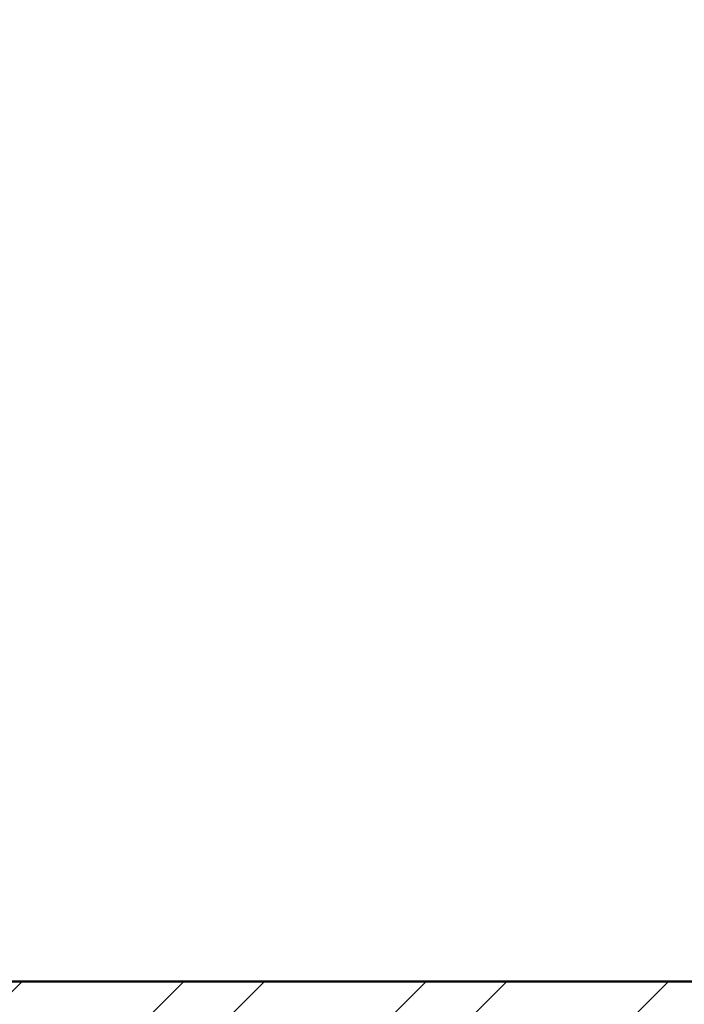
# Model space of a CAD drawing. Units: inches. Extents: x 1901 to 2863, y 888 to 2433.
# Tile 79 of 91: x 2608 to 2645, y 2009 to 2064. Entities that reach past the tile are written whole.
import ezdxf

# ---------------------------------------------------------------- set-up
doc = ezdxf.new("R2010")
doc.units = ezdxf.units.IN
doc.layers.add('A-WALL', color=7, linetype='Continuous', lineweight=50)
doc.layers.add('A-WALL-PATT', color=8, linetype='Continuous', lineweight=13)

msp = doc.modelspace()

# ---------------------------------------------------------------- hatches: boundary and pattern name
at = {"layer": 'A-WALL-PATT'}
h = msp.add_hatch(dxfattribs=at)
h.set_pattern_fill('ANSI32', color=256)
h.paths.add_polyline_path([(2192.501, 2274.134), (2141.264, 2274.134), (2141.264, 2269.634), (2192.501, 2269.634)])
h.paths.add_polyline_path([(2259.926, 2274.134), (2216.501, 2274.134), (2216.501, 2269.634), (2255.426, 2269.634), (2255.426, 2214.634), (2250.809, 2214.634), (2250.809, 2210.134), (2259.926, 2210.134), (2259.926, 2215.134), (2271.756, 2215.134), (2271.756, 2217.384), (2271.756, 2219.634), (2259.926, 2219.634)])
h.paths.add_polyline_path([(2171.426, 2269.634), (2166.926, 2269.634), (2166.926, 2219.634), (2121.238, 2219.634), (2121.238, 2215.134), (2166.926, 2215.134), (2166.926, 2083.134), (2161.807, 2083.134), (2161.807, 2078.634), (2171.426, 2078.634), (2176.996, 2078.634), (2176.996, 2080.884), (2176.996, 2083.134), (2171.426, 2083.134), (2171.426, 2210.134), (2230.912, 2210.134), (2230.912, 2212.384), (2230.912, 2214.634), (2171.426, 2214.634)])
h.paths.add_polyline_path([(2117.264, 2274.134), (2089.426, 2274.134), (2089.426, 2219.634), (2081.136, 2219.634), (2081.136, 2215.134), (2089.426, 2215.134), (2098.004, 2215.134), (2098.004, 2217.384), (2098.004, 2219.634), (2093.926, 2219.634), (2093.926, 2269.634), (2117.264, 2269.634), (2117.264, 2271.884)])
h.paths.add_polyline_path([(2343.426, 2219.634), (2329.295, 2219.634), (2329.295, 2215.134), (2338.926, 2215.134), (2338.926, 2184.739), (2343.426, 2184.739)])
h.paths.add_polyline_path([(2338.926, 2083.134), (2329.295, 2083.134), (2208.966, 2083.134), (2208.966, 2078.634), (2338.926, 2078.634)])
h.paths.add_polyline_path([(2343.426, 2136.739), (2338.926, 2136.739), (2338.926, 1872.634), (2343.426, 1872.634)])
h.paths.add_polyline_path([(2343.426, 1863.634), (2397.68, 1863.634), (2397.68, 1821.634), (2384.138, 1821.634), (2384.138, 1812.634), (2418.33, 1812.634), (2418.33, 1817.134), (2418.33, 1821.634), (2406.68, 1821.634), (2406.68, 1863.634), (2459.499, 1863.634), (2459.499, 1821.634), (2447.138, 1821.634), (2447.138, 1812.634), (2459.499, 1812.634), (2468.499, 1812.634), (2468.499, 1872.634), (2394.426, 1872.634), (2334.426, 1872.634), (2334.426, 1812.634), (2343.426, 1812.634), (2353.251, 1812.634), (2353.251, 1821.634), (2343.426, 1821.634)])
h.paths.add_polyline_path([(2510.014, 1872.634), (2468.499, 1872.634), (2468.499, 1868.134), (2510.014, 1868.134)])
h.paths.add_polyline_path([(2514.009, 1817.134), (2468.499, 1817.134), (2468.499, 1812.634), (2482.114, 1812.634), (2482.114, 1800.606), (2486.614, 1800.606), (2486.614, 1812.634), (2514.009, 1812.634)])
h.paths.add_polyline_path([(2299.247, 1814.884), (2299.247, 1817.134), (2295.926, 1817.134), (2295.926, 1854.169), (2293.676, 1854.169), (2291.426, 1854.169), (2291.426, 1817.134), (2266.109, 1817.134), (2266.109, 1812.634), (2299.247, 1812.634)])
h.paths.add_polyline_path([(2218.109, 1817.134), (2206.46, 1817.134), (2171.426, 1817.134), (2171.426, 1949.134), (2190.1, 1949.134), (2190.1, 1953.634), (2163.468, 1953.634), (2163.468, 1949.134), (2166.926, 1949.134), (2166.926, 1817.134), (2114.297, 1817.134), (2114.297, 1812.634), (2218.109, 1812.634)])
h.paths.add_polyline_path([(2029.426, 1970.922), (2024.926, 1970.922), (2024.926, 1912.717), (2029.426, 1912.717)])
h.paths.add_polyline_path([(2132.297, 1953.634), (2113.926, 1953.634), (2113.926, 1975.888), (2111.676, 1975.888), (2109.426, 1975.888), (2109.426, 1953.634), (2029.426, 1953.634), (2029.426, 1949.134), (2132.297, 1949.134)])
h.paths.add_polyline_path([(2029.426, 1853.606), (2029.31, 1853.606), (2029.31, 1853.606), (2029.426, 1853.606), (2029.426, 1864.717), (2024.926, 1864.717), (2024.926, 1812.634), (2066.297, 1812.634), (2066.297, 1814.884), (2066.297, 1817.134), (2029.426, 1817.134)])
h.paths.add_polyline_path([(2122.926, 2010.088), (2120.676, 2010.088), (2118.426, 2010.088), (2118.426, 2006.134), (2029.426, 2006.134), (2029.426, 2001.634), (2109.426, 2001.634), (2109.426, 1998.041), (2113.926, 1998.041), (2113.926, 2001.634), (2122.926, 2001.634)])
h.paths.add_polyline_path([(2029.426, 2031.376), (2024.926, 2031.376), (2024.926, 1994.922), (2027.176, 1994.922), (2029.426, 1994.922)])
h.paths.add_polyline_path([(2029.426, 2136.739), (2024.926, 2136.739), (2024.926, 2067.376), (2027.176, 2067.376), (2029.426, 2067.376)])
h.paths.add_polyline_path([(2125.618, 2083.134), (2029.426, 2083.134), (2029.426, 2078.634), (2118.426, 2078.634), (2118.426, 2030.715), (2122.926, 2030.715), (2122.926, 2078.634), (2125.618, 2078.634)])
h.paths.add_polyline_path([(2029.426, 2215.134), (2040.468, 2215.134), (2040.468, 2217.384), (2040.468, 2219.634), (2024.926, 2219.634), (2024.926, 2184.739), (2029.426, 2184.739), (2029.426, 2187.778)])
h.paths.add_polyline_path([(2686.426, 2274.134), (2659.284, 2274.134), (2659.284, 2269.634), (2681.926, 2269.634), (2681.926, 2219.634), (2676.816, 2219.634), (2676.816, 2215.134), (2681.926, 2215.134), (2697.011, 2215.134), (2697.011, 2217.384), (2697.011, 2219.634), (2686.426, 2219.634)])
h.paths.add_polyline_path([(2609.926, 2269.634), (2635.284, 2269.634), (2635.284, 2274.134), (2571.431, 2274.134), (2571.431, 2269.634), (2605.426, 2269.634), (2605.426, 2214.634), (2549.098, 2214.634), (2549.098, 2210.134), (2605.426, 2210.134), (2605.426, 2083.134), (2601.014, 2083.134), (2601.014, 2080.884), (2601.014, 2078.634), (2609.926, 2078.634), (2616.162, 2078.634), (2616.162, 2080.884), (2616.162, 2083.134), (2609.926, 2083.134), (2609.926, 2215.134), (2651.465, 2215.134), (2651.465, 2217.384), (2651.465, 2219.634), (2609.926, 2219.634)])
h.paths.add_polyline_path([(2521.426, 2269.634), (2547.431, 2269.634), (2547.431, 2271.884), (2547.431, 2274.134), (2516.926, 2274.134), (2516.926, 2219.634), (2506.41, 2219.634), (2506.41, 2215.134), (2516.926, 2215.134), (2516.926, 2210.134), (2525.402, 2210.134), (2525.402, 2212.384), (2525.402, 2214.634), (2521.426, 2214.634)])
h.paths.add_polyline_path([(2456.011, 2219.634), (2439.426, 2219.634), (2439.426, 2187.888), (2443.926, 2187.888), (2443.926, 2215.134), (2456.011, 2215.134)])
h.paths.add_polyline_path([(2752.926, 2219.634), (2739.485, 2219.634), (2739.485, 2215.134), (2748.426, 2215.134), (2748.426, 2187.888), (2752.926, 2187.888)])
h.paths.add_polyline_path([(2752.926, 2139.888), (2748.426, 2139.888), (2748.426, 2083.134), (2648.416, 2083.134), (2648.416, 2078.634), (2654.926, 2078.634), (2654.926, 2039.437), (2659.426, 2039.437), (2659.426, 2078.634), (2748.426, 2078.634), (2748.426, 2063.429), (2752.926, 2063.429)])
h.paths.add_polyline_path([(2752.926, 2010.634), (2659.426, 2010.634), (2659.426, 2015.652), (2654.926, 2015.652), (2654.926, 2010.634), (2605.426, 2010.634), (2605.426, 1920.967), (2609.926, 1920.967), (2609.926, 2006.134), (2748.426, 2006.134), (2748.426, 1982.466), (2752.926, 1982.466)])
h.paths.add_polyline_path([(2752.926, 2027.429), (2748.426, 2027.429), (2748.426, 2010.634), (2752.926, 2010.634)])
h.paths.add_polyline_path([(2748.426, 1886.134), (2609.926, 1886.134), (2609.926, 1889.719), (2605.426, 1889.719), (2605.426, 1861.262), (2609.926, 1861.262), (2609.926, 1881.634), (2748.426, 1881.634)])
h.paths.add_polyline_path([(2456.855, 2228.831), (2498.401, 2228.831), (2498.401, 2247.488), (2456.855, 2247.488)], flags=9)
h.paths.add_polyline_path([(2038.602, 2237.418), (2080.174, 2237.418), (2080.174, 2256.075), (2038.602, 2256.075)], flags=9)
h.paths.add_polyline_path([(2292.009, 1062.394), (2539.932, 1062.394), (2539.932, 1099.487), (2292.009, 1099.487)], flags=9)
h.paths.add_polyline_path([(2424.91, 1832.253), (2448.513, 1832.253), (2448.513, 1846.678), (2424.91, 1846.678)], flags=25)
h.paths.add_polyline_path([(2359.076, 1832.253), (2382.678, 1832.253), (2382.678, 1846.678), (2359.076, 1846.678)], flags=25)
h.paths.add_polyline_path([(2352.899, 1684.802), (2367.543, 1684.802), (2367.543, 1697.167), (2352.899, 1697.167)], flags=9)
h.paths.add_polyline_path([(2079.288, 1755.826), (2169.024, 1755.826), (2169.024, 1774.372), (2079.288, 1774.372)], flags=9)
h.paths.add_polyline_path([(2404.09, 1373.857), (2404.09, 1463.593), (2385.544, 1463.593), (2385.544, 1373.857)], flags=9)
h.paths.add_polyline_path([(2268.091, 2236.371), (2309.636, 2236.371), (2309.636, 2255.028), (2268.091, 2255.028)], flags=9)
h.paths.add_polyline_path([(2575.96, 1700.951), (2665.696, 1700.951), (2665.696, 1719.498), (2575.96, 1719.498)], flags=9)
h.paths.add_polyline_path([(2302.962, 1878.474), (2329.524, 1878.474), (2329.524, 1888.777), (2302.962, 1888.777)], flags=9)
h.paths.add_polyline_path([(2097.415, 2240.576), (2126.573, 2240.576), (2126.573, 2259.233), (2097.415, 2259.233)], flags=9)
h.paths.add_polyline_path([(2208.725, 2246.124), (2237.882, 2246.124), (2237.882, 2264.781), (2208.725, 2264.781)], flags=9)
h.paths.add_polyline_path([(2038.147, 1925.958), (2076.987, 1925.958), (2076.987, 1944.615), (2038.147, 1944.615)], flags=9)
h.paths.add_polyline_path([(2239.144, 1926.672), (2288.465, 1926.672), (2288.465, 1945.329), (2239.144, 1945.329)], flags=9)
h.paths.add_polyline_path([(2175.429, 2007.33), (2212.356, 2007.33), (2212.356, 2025.987), (2175.429, 2025.987)], flags=9)
h.paths.add_polyline_path([(2225.034, 2091.794), (2263.875, 2091.794), (2263.875, 2110.451), (2225.034, 2110.451)], flags=9)
h.paths.add_polyline_path([(2035.398, 2098.478), (2074.238, 2098.478), (2074.238, 2117.135), (2035.398, 2117.135)], flags=9)
h.paths.add_polyline_path([(2050.102, 2029.209), (2083.26, 2029.209), (2083.26, 2047.866), (2050.102, 2047.866)], flags=9)
h.paths.add_polyline_path([(2069.677, 1956.719), (2098.835, 1956.719), (2098.835, 1975.376), (2069.677, 1975.376)], flags=25)
h.paths.add_polyline_path([(2328.62, 1753.336), (2361.663, 1753.336), (2361.663, 1771.993), (2328.62, 1771.993)], flags=9)
h.paths.add_polyline_path([(2395.162, 2060.888), (2395.162, 2140.654), (2378.676, 2140.654), (2378.676, 2060.888)], flags=9)
h.paths.add_polyline_path([(2463.728, 2059.02), (2492.886, 2059.02), (2492.886, 2077.677), (2463.728, 2077.677)], flags=9)
h.paths.add_polyline_path([(2458.027, 2181.536), (2496.868, 2181.536), (2496.868, 2200.194), (2458.027, 2200.194)], flags=9)
h.paths.add_polyline_path([(2527.577, 2243.074), (2556.735, 2243.074), (2556.735, 2261.731), (2527.577, 2261.731)], flags=9)
h.paths.add_polyline_path([(2694.461, 2232.767), (2736.033, 2232.767), (2736.033, 2251.425), (2694.461, 2251.425)], flags=9)
h.paths.add_polyline_path([(2637.821, 2249.225), (2666.979, 2249.225), (2666.979, 2267.882), (2637.821, 2267.882)], flags=9)
h.paths.add_polyline_path([(2623.687, 2183.541), (2662.528, 2183.541), (2662.528, 2202.199), (2623.687, 2202.199)], flags=9)
h.paths.add_polyline_path([(2691.965, 2021.5), (2725.124, 2021.5), (2725.124, 2040.157), (2691.965, 2040.157)], flags=9)
h.paths.add_polyline_path([(2621.043, 1975.912), (2662.335, 1975.912), (2662.335, 1994.569), (2621.043, 1994.569)], flags=25)
h.paths.add_polyline_path([(2479.032, 1927.62), (2519.844, 1927.62), (2519.844, 1946.277), (2479.032, 1946.277)], flags=9)
h.paths.add_polyline_path([(2670.941, 1849.076), (2716.005, 1849.076), (2716.005, 1867.734), (2670.941, 1867.734)], flags=9)
h.paths.add_polyline_path([(2523.613, 1782.956), (2550.175, 1782.956), (2550.175, 1793.26), (2523.613, 1793.26)], flags=9)
h.paths.add_polyline_path([(2450.841, 1207.331), (2492.386, 1207.331), (2492.386, 1225.989), (2450.841, 1225.989)], flags=9)
h.paths.add_polyline_path([(2527.751, 1203.841), (2556.908, 1203.841), (2556.908, 1222.499), (2527.751, 1222.499)], flags=9)
h.paths.add_polyline_path([(2639.111, 1207.2), (2668.268, 1207.2), (2668.268, 1225.857), (2639.111, 1225.857)], flags=9)
h.paths.add_polyline_path([(2692.594, 1218.965), (2734.167, 1218.965), (2734.167, 1237.623), (2692.594, 1237.623)], flags=9)
h.paths.add_polyline_path([(2669.266, 1366.329), (2708.106, 1366.329), (2708.106, 1384.987), (2669.266, 1384.987)], flags=9)
h.paths.add_polyline_path([(2463.313, 1358.031), (2502.153, 1358.031), (2502.153, 1376.688), (2463.313, 1376.688)], flags=9)
h.paths.add_polyline_path([(2494.725, 1449.963), (2531.652, 1449.963), (2531.652, 1468.62), (2494.725, 1468.62)], flags=9)
h.paths.add_polyline_path([(2675.565, 1422.157), (2708.724, 1422.157), (2708.724, 1440.815), (2675.565, 1440.815)], flags=9)
h.paths.add_polyline_path([(2685.634, 1493.891), (2714.792, 1493.891), (2714.792, 1512.548), (2685.634, 1512.548)], flags=9)
h.paths.add_polyline_path([(2686.805, 1529.913), (2725.645, 1529.913), (2725.645, 1548.57), (2686.805, 1548.57)], flags=9)
h.paths.add_polyline_path([(2503.651, 1537.991), (2552.972, 1537.991), (2552.972, 1556.648), (2503.651, 1556.648)], flags=9)
h.paths.add_polyline_path([(2291.713, 1643.504), (2318.275, 1643.504), (2318.275, 1653.807), (2291.713, 1653.807)], flags=9)
h.paths.add_polyline_path([(2450.626, 1610.52), (2477.189, 1610.52), (2477.189, 1620.824), (2450.626, 1620.824)], flags=9)
h.paths.add_polyline_path([(2359.985, 1551.814), (2422.253, 1551.814), (2422.253, 1562.117), (2359.985, 1562.117)], flags=9)
h.paths.add_polyline_path([(2280.106, 1249.006), (2321.651, 1249.006), (2321.651, 1267.663), (2280.106, 1267.663)], flags=9)
h.paths.add_polyline_path([(2164.057, 1274.232), (2193.215, 1274.232), (2193.215, 1292.889), (2164.057, 1292.889)], flags=9)
h.paths.add_polyline_path([(2118.21, 1277.694), (2151.252, 1277.694), (2151.252, 1296.351), (2118.21, 1296.351)], flags=9)
h.paths.add_polyline_path([(2031.946, 1268.529), (2073.519, 1268.529), (2073.519, 1287.187), (2031.946, 1287.187)], flags=9)
h.paths.add_polyline_path([(2050.199, 1409.079), (2089.04, 1409.079), (2089.04, 1427.736), (2050.199, 1427.736)], flags=9)
h.paths.add_polyline_path([(2243.743, 1421.032), (2282.584, 1421.032), (2282.584, 1439.689), (2243.743, 1439.689)], flags=9)
h.paths.add_polyline_path([(2190.746, 1509.769), (2231.558, 1509.769), (2231.558, 1528.426), (2190.746, 1528.426)], flags=9)
h.paths.add_polyline_path([(2058.392, 1475.415), (2091.55, 1475.415), (2091.55, 1494.073), (2058.392, 1494.073)], flags=9)
h.paths.add_polyline_path([(2062.447, 1553.09), (2091.605, 1553.09), (2091.605, 1571.747), (2062.447, 1571.747)], flags=9)
h.paths.add_polyline_path([(2219.524, 1590.365), (2266.147, 1590.365), (2266.147, 1609.022), (2219.524, 1609.022)], flags=9)
h.paths.add_polyline_path([(2041.072, 1584.188), (2079.912, 1584.188), (2079.912, 1602.845), (2041.072, 1602.845)], flags=9)

# ---------------------------------------------------------------- linework, layer by layer
at = {"layer": 'A-WALL'}
msp.add_line((2654.926, 2010.634), (2605.426, 2010.634), dxfattribs=at)

doc.saveas('drawing.dxf')
